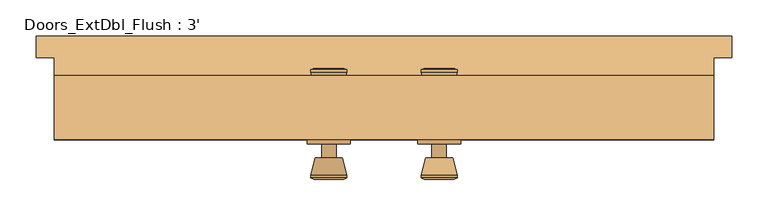
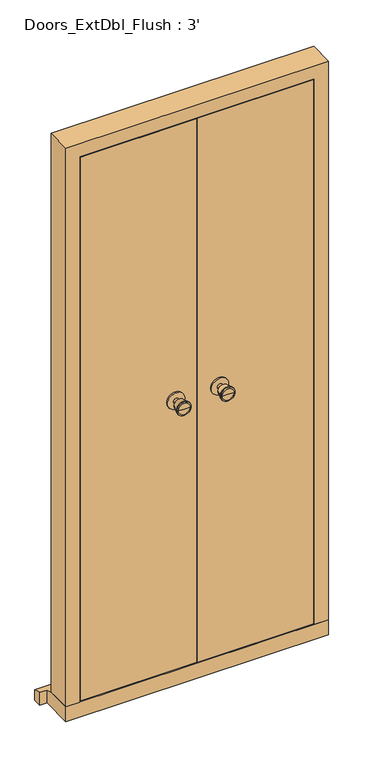
"""IFC4 building model written with IfcOpenShell, lengths in millimetres: door geometry, Doors_ExtDbl_Flush : 3'."""

from ifc_helpers import new_model, si_unit, point, frame, frame_2d, origin, place, context, project, spatial, polyline, circle_curve, trimmed, segment, composite_curve, outline, extrude, faceted_brep, source, transform, mapped, element, save
from ifc_brep_helpers import plane_surface, cylinder_surface, revolved_surface, advanced_brep


def doors_extdbl_flush_3_b8e651f3(model_context):
    return source(origin(), model_context, "Body", "SolidModel", [
        advanced_brep(
        [(-76.5, -43.8, 1050.0), (-66.5, -43.8, 1050.0), (-86.5, -43.8, 1050.0), (-96.9758676, -92.8, 1050.0), (-56.0241324, -92.8, 1050.0), (-76.5, -92.8, 1050.0), (-101.5, -90.9721319, 1050.0), (-51.5, -90.9721319, 1050.0), (-101.5, -87.5084537, 1050.0), (-51.5, -87.5084537, 1050.0), (-95.136236, -62.8, 1050.0), (-57.863764, -62.8, 1050.0), (-86.5, -62.8, 1050.0), (-66.5, -62.8, 1050.0)],
        [
            (0, 1),
            (1, 2, circle_curve(frame((-76.5, -43.8, 1050.0), z_axis=(0.0, 1.0, 0.0), x_axis=(1.0, 0.0, 0.0)), 10.0)),
            (2, 0),
            (2, 1, circle_curve(frame((-76.5, -43.8, 1050.0), z_axis=(0.0, 1.0, 0.0), x_axis=(1.0, 0.0, 0.0)), 10.0)),
            (3, 4, circle_curve(frame((-76.5, -92.8, 1050.0), z_axis=(0.0, -1.0, 0.0), x_axis=(1.0, 0.0, 0.0)), 20.4758676)),
            (4, 5),
            (5, 3),
            (4, 3, circle_curve(frame((-76.5, -92.8, 1050.0), z_axis=(0.0, -1.0, 0.0), x_axis=(1.0, 0.0, 0.0)), 20.4758676)),
            (6, 7, circle_curve(frame((-76.5, -90.9721319, 1050.0), z_axis=(0.0, -1.0, 0.0), x_axis=(1.0, 0.0, 0.0)), 25.0)),
            (7, 4),
            (3, 6),
            (7, 6, circle_curve(frame((-76.5, -90.9721319, 1050.0), z_axis=(0.0, -1.0, 0.0), x_axis=(1.0, 0.0, 0.0)), 25.0)),
            (8, 9, circle_curve(frame((-76.5, -87.5084537, 1050.0), z_axis=(0.0, -1.0, 0.0), x_axis=(1.0, 0.0, 0.0)), 25.0)),
            (9, 7),
            (6, 8),
            (9, 8, circle_curve(frame((-76.5, -87.5084537, 1050.0), z_axis=(0.0, -1.0, 0.0), x_axis=(1.0, 0.0, 0.0)), 25.0)),
            (10, 11, circle_curve(frame((-76.5, -62.8, 1050.0), z_axis=(0.0, -1.0, 0.0), x_axis=(1.0, 0.0, 0.0)), 18.636236)),
            (11, 9),
            (8, 10),
            (11, 10, circle_curve(frame((-76.5, -62.8, 1050.0), z_axis=(0.0, -1.0, 0.0), x_axis=(1.0, 0.0, 0.0)), 18.636236)),
            (12, 13, circle_curve(frame((-76.5, -62.8, 1050.0), z_axis=(0.0, -1.0, 0.0), x_axis=(1.0, 0.0, 0.0)), 10.0)),
            (13, 11),
            (10, 12),
            (13, 12, circle_curve(frame((-76.5, -62.8, 1050.0), z_axis=(0.0, -1.0, 0.0), x_axis=(1.0, 0.0, 0.0)), 10.0)),
            (1, 13),
            (12, 2),
        ],
        [
            plane_surface(frame((-76.5, -43.8, 1050.0), z_axis=(0.0, 1.0, 0.0), x_axis=(1.0, 0.0, 0.0))),
            plane_surface(frame((-76.5, -92.8, 1050.0), z_axis=(0.0, -1.0, 0.0), x_axis=(1.0, 0.0, 0.0))),
            revolved_surface(polyline([(-56.0241324, -92.8, 1050.0), (-51.5, -90.9721319, 1050.0)]), (-76.5, -43.8, 1050.0), (0.0, 1.0, 0.0)),
            cylinder_surface(frame((-76.5, -43.8, 1050.0), z_axis=(0.0, 1.0, 0.0), x_axis=(1.0, 0.0, 0.0)), 25.0),
            revolved_surface(polyline([(-51.5, -87.5084537, 1050.0), (-57.863764, -62.8, 1050.0)]), (-76.5, -43.8, 1050.0), (0.0, 1.0, 0.0)),
            plane_surface(frame((-76.5, -62.8, 1050.0), z_axis=(0.0, 1.0, 0.0), x_axis=(1.0, 0.0, 0.0))),
            cylinder_surface(frame((-76.5, -43.8, 1050.0), z_axis=(0.0, 1.0, 0.0), x_axis=(1.0, 0.0, 0.0)), 10.0),
        ],
        [
            (0, [[1, 2, 3]]),
            (0, [[-3, 4, -1]]),
            (1, [[5, 6, 7]]),
            (1, [[8, -7, -6]]),
            (2, [[9, 10, -5, 11]]),
            (2, [[12, -11, -8, -10]]),
            (3, [[13, 14, -9, 15]]),
            (3, [[16, -15, -12, -14]]),
            (4, [[17, 18, -13, 19]]),
            (4, [[20, -19, -16, -18]]),
            (5, [[21, 22, -17, 23]]),
            (5, [[24, -23, -20, -22]]),
            (6, [[-2, 25, -21, 26]]),
            (6, [[-4, -26, -24, -25]]),
        ],
    ),
        extrude(outline(composite_curve([segment(trimmed(circle_curve(frame_2d((1050.0, -76.5)), 30.0), [point((1050.0, -46.5))], [point((1050.0, -106.5))], False, "CARTESIAN"), True, "CONTINUOUS"), segment(trimmed(circle_curve(frame_2d((1050.0, -76.5)), 30.0), [point((1050.0, -106.5))], [point((1050.0, -46.5))], False, "CARTESIAN"), True, "CONTINUOUS")], self_intersect=False)), frame((0.0, -43.8, 0.0), z_axis=(0.0, 1.0, 0.0), x_axis=(0.0, 0.0, 1.0)), (0.0, 0.0, 1.0), 6.0),
        advanced_brep(
        [(-76.5, 12.2, 1050.0), (-86.5, 12.2, 1050.0), (-66.5, 12.2, 1050.0), (-96.9758676, 61.2, 1050.0), (-76.5, 61.2, 1050.0), (-56.0241324, 61.2, 1050.0), (-101.5, 59.3721319, 1050.0), (-51.5, 59.3721319, 1050.0), (-101.5, 55.9084537, 1050.0), (-51.5, 55.9084537, 1050.0), (-95.136236, 31.2, 1050.0), (-57.863764, 31.2, 1050.0), (-86.5, 31.2, 1050.0), (-66.5, 31.2, 1050.0)],
        [
            (0, 1),
            (1, 2, circle_curve(frame((-76.5, 12.2, 1050.0), z_axis=(0.0, -1.0, 0.0), x_axis=(1.0, 0.0, 0.0)), 10.0)),
            (2, 0),
            (2, 1, circle_curve(frame((-76.5, 12.2, 1050.0), z_axis=(0.0, -1.0, 0.0), x_axis=(1.0, 0.0, 0.0)), 10.0)),
            (3, 4),
            (4, 5),
            (5, 3, circle_curve(frame((-76.5, 61.2, 1050.0), z_axis=(0.0, 1.0, 0.0), x_axis=(1.0, 0.0, 0.0)), 20.4758676)),
            (3, 5, circle_curve(frame((-76.5, 61.2, 1050.0), z_axis=(0.0, 1.0, 0.0), x_axis=(1.0, 0.0, 0.0)), 20.4758676)),
            (6, 3),
            (5, 7),
            (7, 6, circle_curve(frame((-76.5, 59.3721319, 1050.0), z_axis=(0.0, 1.0, 0.0), x_axis=(1.0, 0.0, 0.0)), 25.0)),
            (6, 7, circle_curve(frame((-76.5, 59.3721319, 1050.0), z_axis=(0.0, 1.0, 0.0), x_axis=(1.0, 0.0, 0.0)), 25.0)),
            (8, 6),
            (7, 9),
            (9, 8, circle_curve(frame((-76.5, 55.9084537, 1050.0), z_axis=(0.0, 1.0, 0.0), x_axis=(1.0, 0.0, 0.0)), 25.0)),
            (8, 9, circle_curve(frame((-76.5, 55.9084537, 1050.0), z_axis=(0.0, 1.0, 0.0), x_axis=(1.0, 0.0, 0.0)), 25.0)),
            (10, 8),
            (9, 11),
            (11, 10, circle_curve(frame((-76.5, 31.2, 1050.0), z_axis=(0.0, 1.0, 0.0), x_axis=(1.0, 0.0, 0.0)), 18.636236)),
            (10, 11, circle_curve(frame((-76.5, 31.2, 1050.0), z_axis=(0.0, 1.0, 0.0), x_axis=(1.0, 0.0, 0.0)), 18.636236)),
            (12, 10),
            (11, 13),
            (13, 12, circle_curve(frame((-76.5, 31.2, 1050.0), z_axis=(0.0, 1.0, 0.0), x_axis=(1.0, 0.0, 0.0)), 10.0)),
            (12, 13, circle_curve(frame((-76.5, 31.2, 1050.0), z_axis=(0.0, 1.0, 0.0), x_axis=(1.0, 0.0, 0.0)), 10.0)),
            (1, 12),
            (13, 2),
        ],
        [
            plane_surface(frame((-76.5, 12.2, 1050.0), z_axis=(0.0, -1.0, 0.0), x_axis=(1.0, 0.0, 0.0))),
            plane_surface(frame((-76.5, 61.2, 1050.0), z_axis=(0.0, 1.0, 0.0), x_axis=(1.0, 0.0, 0.0))),
            revolved_surface(polyline([(-56.0241324, 61.2, 1050.0), (-51.5, 59.3721319, 1050.0)]), (-76.5, 12.2, 1050.0), (0.0, -1.0, 0.0)),
            cylinder_surface(frame((-76.5, 12.2, 1050.0), z_axis=(0.0, -1.0, 0.0), x_axis=(1.0, 0.0, 0.0)), 25.0),
            revolved_surface(polyline([(-51.5, 55.9084537, 1050.0), (-57.863764, 31.2, 1050.0)]), (-76.5, 12.2, 1050.0), (0.0, -1.0, 0.0)),
            plane_surface(frame((-76.5, 31.2, 1050.0), z_axis=(0.0, -1.0, 0.0), x_axis=(1.0, 0.0, 0.0))),
            cylinder_surface(frame((-76.5, 12.2, 1050.0), z_axis=(0.0, -1.0, 0.0), x_axis=(1.0, 0.0, 0.0)), 10.0),
        ],
        [
            (0, [[1, 2, 3]]),
            (0, [[-3, 4, -1]]),
            (1, [[5, 6, 7]]),
            (1, [[-6, -5, 8]]),
            (2, [[9, -7, 10, 11]]),
            (2, [[-10, -8, -9, 12]]),
            (3, [[13, -11, 14, 15]]),
            (3, [[-14, -12, -13, 16]]),
            (4, [[17, -15, 18, 19]]),
            (4, [[-18, -16, -17, 20]]),
            (5, [[21, -19, 22, 23]]),
            (5, [[-22, -20, -21, 24]]),
            (6, [[25, -23, 26, -2]]),
            (6, [[-26, -24, -25, -4]]),
        ],
    ),
        extrude(outline(composite_curve([segment(trimmed(circle_curve(frame_2d((1050.0, -76.5)), 30.0), [point((1050.0, -46.5))], [point((1050.0, -106.5))], False, "CARTESIAN"), True, "CONTINUOUS"), segment(trimmed(circle_curve(frame_2d((1050.0, -76.5)), 30.0), [point((1050.0, -106.5))], [point((1050.0, -46.5))], False, "CARTESIAN"), True, "CONTINUOUS")], self_intersect=False)), frame((0.0, 6.2, 0.0), z_axis=(0.0, 1.0, 0.0), x_axis=(0.0, 0.0, 1.0)), (0.0, 0.0, 1.0), 6.0),
        advanced_brep(
        [(76.5, -43.8, 1050.0), (86.5, -43.8, 1050.0), (66.5, -43.8, 1050.0), (96.9758676, -92.8, 1050.0), (76.5, -92.8, 1050.0), (56.0241324, -92.8, 1050.0), (101.5, -90.9721319, 1050.0), (51.5, -90.9721319, 1050.0), (101.5, -87.5084537, 1050.0), (51.5, -87.5084537, 1050.0), (95.136236, -62.8, 1050.0), (57.863764, -62.8, 1050.0), (86.5, -62.8, 1050.0), (66.5, -62.8, 1050.0)],
        [
            (0, 1),
            (1, 2, circle_curve(frame((76.5, -43.8, 1050.0), z_axis=(0.0, 1.0, 0.0), x_axis=(-1.0, 0.0, 0.0)), 10.0)),
            (2, 0),
            (2, 1, circle_curve(frame((76.5, -43.8, 1050.0), z_axis=(0.0, 1.0, 0.0), x_axis=(-1.0, 0.0, 0.0)), 10.0)),
            (3, 4),
            (4, 5),
            (5, 3, circle_curve(frame((76.5, -92.8, 1050.0), z_axis=(0.0, -1.0, 0.0), x_axis=(-1.0, 0.0, 0.0)), 20.4758676)),
            (3, 5, circle_curve(frame((76.5, -92.8, 1050.0), z_axis=(0.0, -1.0, 0.0), x_axis=(-1.0, 0.0, 0.0)), 20.4758676)),
            (6, 3),
            (5, 7),
            (7, 6, circle_curve(frame((76.5, -90.9721319, 1050.0), z_axis=(0.0, -1.0, 0.0), x_axis=(-1.0, 0.0, 0.0)), 25.0)),
            (6, 7, circle_curve(frame((76.5, -90.9721319, 1050.0), z_axis=(0.0, -1.0, 0.0), x_axis=(-1.0, 0.0, 0.0)), 25.0)),
            (8, 6),
            (7, 9),
            (9, 8, circle_curve(frame((76.5, -87.5084537, 1050.0), z_axis=(0.0, -1.0, 0.0), x_axis=(-1.0, 0.0, 0.0)), 25.0)),
            (8, 9, circle_curve(frame((76.5, -87.5084537, 1050.0), z_axis=(0.0, -1.0, 0.0), x_axis=(-1.0, 0.0, 0.0)), 25.0)),
            (10, 8),
            (9, 11),
            (11, 10, circle_curve(frame((76.5, -62.8, 1050.0), z_axis=(0.0, -1.0, 0.0), x_axis=(-1.0, 0.0, 0.0)), 18.636236)),
            (10, 11, circle_curve(frame((76.5, -62.8, 1050.0), z_axis=(0.0, -1.0, 0.0), x_axis=(-1.0, 0.0, 0.0)), 18.636236)),
            (12, 10),
            (11, 13),
            (13, 12, circle_curve(frame((76.5, -62.8, 1050.0), z_axis=(0.0, -1.0, 0.0), x_axis=(-1.0, 0.0, 0.0)), 10.0)),
            (12, 13, circle_curve(frame((76.5, -62.8, 1050.0), z_axis=(0.0, -1.0, 0.0), x_axis=(-1.0, 0.0, 0.0)), 10.0)),
            (1, 12),
            (13, 2),
        ],
        [
            plane_surface(frame((76.5, -43.8, 1050.0), z_axis=(0.0, 1.0, 0.0), x_axis=(-1.0, 0.0, 0.0))),
            plane_surface(frame((76.5, -92.8, 1050.0), z_axis=(0.0, -1.0, 0.0), x_axis=(-1.0, 0.0, 0.0))),
            revolved_surface(polyline([(56.0241324, -92.8, 1050.0), (51.5, -90.9721319, 1050.0)]), (76.5, -43.8, 1050.0), (0.0, 1.0, 0.0)),
            cylinder_surface(frame((76.5, -43.8, 1050.0), z_axis=(0.0, 1.0, 0.0), x_axis=(-1.0, 0.0, 0.0)), 25.0),
            revolved_surface(polyline([(51.5, -87.5084537, 1050.0), (57.863764, -62.8, 1050.0)]), (76.5, -43.8, 1050.0), (0.0, 1.0, 0.0)),
            plane_surface(frame((76.5, -62.8, 1050.0), z_axis=(0.0, 1.0, 0.0), x_axis=(-1.0, 0.0, 0.0))),
            cylinder_surface(frame((76.5, -43.8, 1050.0), z_axis=(0.0, 1.0, 0.0), x_axis=(-1.0, 0.0, 0.0)), 10.0),
        ],
        [
            (0, [[1, 2, 3]]),
            (0, [[-3, 4, -1]]),
            (1, [[5, 6, 7]]),
            (1, [[-6, -5, 8]]),
            (2, [[9, -7, 10, 11]]),
            (2, [[-10, -8, -9, 12]]),
            (3, [[13, -11, 14, 15]]),
            (3, [[-14, -12, -13, 16]]),
            (4, [[17, -15, 18, 19]]),
            (4, [[-18, -16, -17, 20]]),
            (5, [[21, -19, 22, 23]]),
            (5, [[-22, -20, -21, 24]]),
            (6, [[25, -23, 26, -2]]),
            (6, [[-26, -24, -25, -4]]),
        ],
    ),
        extrude(outline(composite_curve([segment(trimmed(circle_curve(frame_2d((1050.0, 76.5)), 30.0), [point((1050.0, 46.5))], [point((1050.0, 106.5))], False, "CARTESIAN"), True, "CONTINUOUS"), segment(trimmed(circle_curve(frame_2d((1050.0, 76.5)), 30.0), [point((1050.0, 106.5))], [point((1050.0, 46.5))], False, "CARTESIAN"), True, "CONTINUOUS")], self_intersect=False)), frame((0.0, -43.8, 0.0), z_axis=(0.0, 1.0, 0.0), x_axis=(0.0, 0.0, 1.0)), (0.0, 0.0, 1.0), 6.0),
        advanced_brep(
        [(76.5, 12.2, 1050.0), (66.5, 12.2, 1050.0), (86.5, 12.2, 1050.0), (96.9758676, 61.2, 1050.0), (56.0241324, 61.2, 1050.0), (76.5, 61.2, 1050.0), (101.5, 59.3721319, 1050.0), (51.5, 59.3721319, 1050.0), (101.5, 55.9084537, 1050.0), (51.5, 55.9084537, 1050.0), (95.136236, 31.2, 1050.0), (57.863764, 31.2, 1050.0), (86.5, 31.2, 1050.0), (66.5, 31.2, 1050.0)],
        [
            (0, 1),
            (1, 2, circle_curve(frame((76.5, 12.2, 1050.0), z_axis=(0.0, -1.0, 0.0), x_axis=(-1.0, 0.0, 0.0)), 10.0)),
            (2, 0),
            (2, 1, circle_curve(frame((76.5, 12.2, 1050.0), z_axis=(0.0, -1.0, 0.0), x_axis=(-1.0, 0.0, 0.0)), 10.0)),
            (3, 4, circle_curve(frame((76.5, 61.2, 1050.0), z_axis=(0.0, 1.0, 0.0), x_axis=(-1.0, 0.0, 0.0)), 20.4758676)),
            (4, 5),
            (5, 3),
            (4, 3, circle_curve(frame((76.5, 61.2, 1050.0), z_axis=(0.0, 1.0, 0.0), x_axis=(-1.0, 0.0, 0.0)), 20.4758676)),
            (6, 7, circle_curve(frame((76.5, 59.3721319, 1050.0), z_axis=(0.0, 1.0, 0.0), x_axis=(-1.0, 0.0, 0.0)), 25.0)),
            (7, 4),
            (3, 6),
            (7, 6, circle_curve(frame((76.5, 59.3721319, 1050.0), z_axis=(0.0, 1.0, 0.0), x_axis=(-1.0, 0.0, 0.0)), 25.0)),
            (8, 9, circle_curve(frame((76.5, 55.9084537, 1050.0), z_axis=(0.0, 1.0, 0.0), x_axis=(-1.0, 0.0, 0.0)), 25.0)),
            (9, 7),
            (6, 8),
            (9, 8, circle_curve(frame((76.5, 55.9084537, 1050.0), z_axis=(0.0, 1.0, 0.0), x_axis=(-1.0, 0.0, 0.0)), 25.0)),
            (10, 11, circle_curve(frame((76.5, 31.2, 1050.0), z_axis=(0.0, 1.0, 0.0), x_axis=(-1.0, 0.0, 0.0)), 18.636236)),
            (11, 9),
            (8, 10),
            (11, 10, circle_curve(frame((76.5, 31.2, 1050.0), z_axis=(0.0, 1.0, 0.0), x_axis=(-1.0, 0.0, 0.0)), 18.636236)),
            (12, 13, circle_curve(frame((76.5, 31.2, 1050.0), z_axis=(0.0, 1.0, 0.0), x_axis=(-1.0, 0.0, 0.0)), 10.0)),
            (13, 11),
            (10, 12),
            (13, 12, circle_curve(frame((76.5, 31.2, 1050.0), z_axis=(0.0, 1.0, 0.0), x_axis=(-1.0, 0.0, 0.0)), 10.0)),
            (1, 13),
            (12, 2),
        ],
        [
            plane_surface(frame((76.5, 12.2, 1050.0), z_axis=(0.0, -1.0, 0.0), x_axis=(-1.0, 0.0, 0.0))),
            plane_surface(frame((76.5, 61.2, 1050.0), z_axis=(0.0, 1.0, 0.0), x_axis=(-1.0, 0.0, 0.0))),
            revolved_surface(polyline([(56.0241324, 61.2, 1050.0), (51.5, 59.3721319, 1050.0)]), (76.5, 12.2, 1050.0), (0.0, -1.0, 0.0)),
            cylinder_surface(frame((76.5, 12.2, 1050.0), z_axis=(0.0, -1.0, 0.0), x_axis=(-1.0, 0.0, 0.0)), 25.0),
            revolved_surface(polyline([(51.5, 55.9084537, 1050.0), (57.863764, 31.2, 1050.0)]), (76.5, 12.2, 1050.0), (0.0, -1.0, 0.0)),
            plane_surface(frame((76.5, 31.2, 1050.0), z_axis=(0.0, -1.0, 0.0), x_axis=(-1.0, 0.0, 0.0))),
            cylinder_surface(frame((76.5, 12.2, 1050.0), z_axis=(0.0, -1.0, 0.0), x_axis=(-1.0, 0.0, 0.0)), 10.0),
        ],
        [
            (0, [[1, 2, 3]]),
            (0, [[-3, 4, -1]]),
            (1, [[5, 6, 7]]),
            (1, [[8, -7, -6]]),
            (2, [[9, 10, -5, 11]]),
            (2, [[12, -11, -8, -10]]),
            (3, [[13, 14, -9, 15]]),
            (3, [[16, -15, -12, -14]]),
            (4, [[17, 18, -13, 19]]),
            (4, [[20, -19, -16, -18]]),
            (5, [[21, 22, -17, 23]]),
            (5, [[24, -23, -20, -22]]),
            (6, [[-2, 25, -21, 26]]),
            (6, [[-4, -26, -24, -25]]),
        ],
    ),
        extrude(outline(composite_curve([segment(trimmed(circle_curve(frame_2d((1050.0, 76.5)), 30.0), [point((1050.0, 46.5))], [point((1050.0, 106.5))], False, "CARTESIAN"), True, "CONTINUOUS"), segment(trimmed(circle_curve(frame_2d((1050.0, 76.5)), 30.0), [point((1050.0, 106.5))], [point((1050.0, 46.5))], False, "CARTESIAN"), True, "CONTINUOUS")], self_intersect=False)), frame((0.0, 6.2, 0.0), z_axis=(0.0, 1.0, 0.0), x_axis=(0.0, 0.0, 1.0)), (0.0, 0.0, 1.0), 6.0),
        faceted_brep([(386.7, 51.2, 54.5), (457.2, 51.2, 54.5), (457.2, -37.8, 54.5), (408.7, -37.8, 54.5), (408.7, 9.2, 54.5), (386.7, 9.2, 54.5), (386.7, 51.2, 2039.5), (-386.7, 51.2, 2039.5), (-386.7, 51.2, 54.5), (-457.2, 51.2, 54.5), (-457.2, 51.2, 2110.0), (457.2, 51.2, 2110.0), (457.2, -37.8, 2110.0), (-457.2, -37.8, 2110.0), (-457.2, -37.8, 54.5), (-408.7, -37.8, 54.5), (-408.7, -37.8, 2061.5), (408.7, -37.8, 2061.5), (408.7, 9.2, 2061.5), (-408.7, 9.2, 2061.5), (-408.7, 9.2, 54.5), (-386.7, 9.2, 54.5), (-386.7, 9.2, 2039.5), (386.7, 9.2, 2039.5)], [[[0, 1, 2, 3, 4, 5]], [[1, 0, 6, 7, 8, 9, 10, 11]], [[2, 1, 11, 12]], [[3, 2, 12, 13, 14, 15, 16, 17]], [[4, 3, 17, 18]], [[5, 4, 18, 19, 20, 21, 22, 23]], [[0, 5, 23, 6]], [[7, 22, 21, 8]], [[8, 21, 20, 15, 14, 9]], [[13, 10, 9, 14]], [[19, 16, 15, 20]], [[12, 11, 10, 13]], [[18, 17, 16, 19]], [[6, 23, 22, 7]]]),
        faceted_brep([(482.2, 106.2, 0.0), (482.2, 106.2, 38.5947221), (482.2, 76.2, 47.2703282), (482.2, 76.2, 0.0), (-482.2, 106.2, 38.5947221), (-482.2, 106.2, 0.0), (-482.2, 76.2, 0.0), (-482.2, 76.2, 47.2703282), (457.2, 76.2, 0.0), (457.2, -37.8, 0.0), (-457.2, -37.8, 0.0), (-457.2, 76.2, 0.0), (-457.2, 76.2, 47.2703282), (-457.2, 51.2, 54.5), (457.2, 51.2, 54.5), (457.2, 76.2, 47.2703282), (-457.2, -37.8, 54.5), (457.2, -37.8, 54.5)], [[[0, 1, 2, 3]], [[4, 5, 6, 7]], [[5, 0, 3, 8, 9, 10, 11, 6]], [[1, 0, 5, 4]], [[1, 4, 7, 12, 13, 14, 15, 2]], [[13, 16, 17, 14]], [[16, 10, 9, 17]], [[12, 11, 10, 16, 13]], [[11, 12, 7, 6]], [[8, 15, 14, 17, 9]], [[15, 8, 3, 2]]]),
        extrude(outline(polyline([(405.7, -37.8), (1.5, -37.8), (1.5, 6.2), (405.7, 6.2), (405.7, -37.8)])), frame((0.0, 0.0, 58.5), z_axis=(0.0, 0.0, 1.0), x_axis=(1.0, 0.0, 0.0)), (0.0, 0.0, 1.0), 2000.0),
        extrude(outline(polyline([(-1.5, -37.8), (-405.7, -37.8), (-405.7, 6.2), (-1.5, 6.2), (-1.5, -37.8)])), frame((0.0, 0.0, 58.5), z_axis=(0.0, 0.0, 1.0), x_axis=(1.0, 0.0, 0.0)), (0.0, 0.0, 1.0), 2000.0),
    ])


if __name__ == "__main__":
    model = new_model("IFC4")
    model_context = context("Model", 3, world=origin())
    ifc_project = project(units=[si_unit("LENGTHUNIT", "METRE", prefix="MILLI")], contexts=[model_context])
    site = spatial("IfcSite", under=ifc_project)
    building = spatial("IfcBuilding", under=site)
    placement = place(None, origin())
    doors_extdbl_flush_3_shape = doors_extdbl_flush_3_b8e651f3(model_context)
    element("IfcDoor", 1, ObjectType="Doors_ExtDbl_Flush : 3'", at=placement, inside=building, context=model_context, shape_type="MappedRepresentation", body=[
        mapped(doors_extdbl_flush_3_shape, transform((0.0, 0.0, 0.0), x_axis=(1.0, 0.0, 0.0), y_axis=(0.0, 1.0, 0.0), z_axis=(0.0, 0.0, 1.0))),
    ])
    save(model, "model.ifc")

# Revit data of these elements
# Type "Doors_ExtDbl_Flush : 3'"
#   Type Mark = "55"
#   Type Comments = "External Double"
#   Operation = "DoubleDoorSingleSwing"
#   Keynote = "L20"
#   Analytic Construction = "Metal"
#   Wrap Layers (Ext) from Ext = 102.5 mm
#   Wrap Layers (Int) from Ext = 177.5 mm
#   Thickness = 44 mm
#   Rough Width = 914.4 mm
#   Rough Height = 2110 mm
#   O/A Frame Width = 64 mm
#   Heat Transfer Coefficient (U) = 3.7021 W/(m²·K)
#   Handle Z Distance = 1050 mm
#   FrameWidth = 42 mm
#   FrameOffset - External = 25 mm
#   FrameDepth = 89 mm
#   Door Panel Width = 404.2 mm
#   Door Panel Thickness = 44 mm
#   Door Panel Height = 2000 mm
#   Cill Thickness = 54.5 mm
#   Cill Projection = 30 mm
#   Handle X Distance = 75 mm
#   Height = 2110 mm
#   Structural Tolerance = 6.5 mm
#   Tolerance = 3 mm
#   Undercut = 4 mm
#   Width = 914.4 mm
#   Cill Extension = 25 mm
#   Cavity Closer Width = 50 mm
#   Cavity Closer Offset from Ext = 102.5 mm
#   Cavity Closer Depth = 85 mm
#   Vis - Ironmongery = yes
#   Vis - Cavity Closers = yes
#   Function = 1
#   Material Door = Door - Panel
#   Material Frame = Door - Frame/Mullion
#   Material Ironmongery = Door - Handle
#   Visual Light Transmittance = 0
#   Thermal Resistance (R) = 0
#   Solar Heat Gain Coefficient = 0
#   Wall Closure = (empty or 0)
# Element 1 (IfcDoor, "Doors_ExtDbl_Flush : 3'")
#   Materials on its faces: "Door - Handle", "Door - Frame/Mullion", "Door - Panel"
# Materials
#   "Door - Panel": class "Wood", colour RGB 210 159 95, transparency 0, Keynote = "L20", Cost = 0
#   "Door - Frame/Mullion": class "Wood", colour RGB 212 179 113, transparency 0, Keynote = "L20", Cost = 0
#   "Door - Handle": colour RGB 0 0 0, transparency 0, Keynote = "P21", Cost = 0
